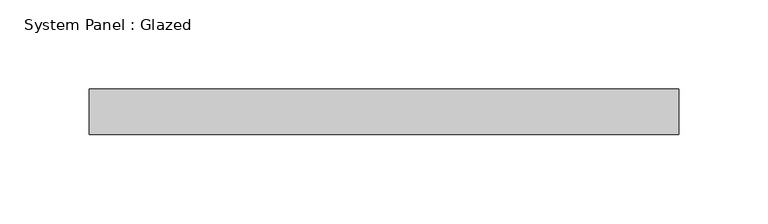
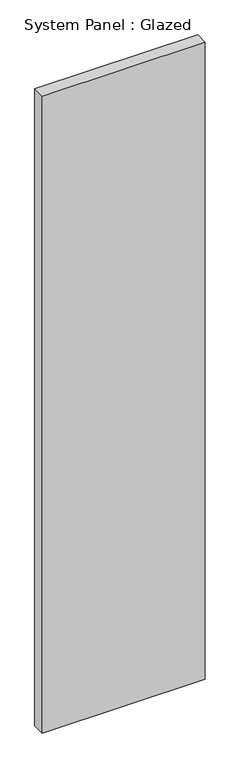
"""IFC4 building model written with IfcOpenShell, lengths in millimetres: plate geometry, System Panel : Glazed."""

from ifc_helpers import new_model, si_unit, origin, origin_with_axes, place, context, project, spatial, polyline, outline, extrude, source, transform, mapped, element, save


def system_panel_glazed_df80ca6a(model_context):
    return source(origin(), model_context, "Body", "SweptSolid", [
        extrude(outline(polyline([(165.1, 19.05), (-165.1, 19.05), (-165.1, 44.45), (165.1, 44.45), (165.1, 19.05)])), origin_with_axes(), (0.0, 0.0, 1.0), 1363.0142793),
    ])


if __name__ == "__main__":
    model = new_model("IFC4")
    model_context = context("Model", 3, world=origin())
    ifc_project = project(units=[si_unit("LENGTHUNIT", "METRE", prefix="MILLI")], contexts=[model_context])
    site = spatial("IfcSite", under=ifc_project)
    building = spatial("IfcBuilding", under=site)
    placement = place(None, origin())
    system_panel_glazed_shape = system_panel_glazed_df80ca6a(model_context)
    element("IfcPlate", 1, ObjectType="System Panel : Glazed", at=placement, inside=building, context=model_context, shape_type="MappedRepresentation", body=[
        mapped(system_panel_glazed_shape, transform((0.0, 0.0, 0.0), x_axis=(1.0, 0.0, 0.0), y_axis=(0.0, 1.0, 0.0), z_axis=(0.0, 0.0, 1.0))),
    ])
    save(model, "model.ifc")

# Revit data of these elements
# Type "System Panel : Glazed"
#   Construction Type Id = "GSP4R"
#   Analytic Construction = "1/8 in Pilkington single glazing"
#   Visual Light Transmittance = 0.9
#   Solar Heat Gain Coefficient = 0.86
#   Heat Transfer Coefficient (U) = 1.18115 BTU/(h·ft²·°F)
#   Define Thermal Properties by = 1
# Element 1 (IfcPlate, "System Panel : Glazed")
#   Materials on its faces: "Glass"
# Materials
#   "Glass": class "Glass", colour RGB 0 128 192, transparency 0.75, Description = "Soda Lime Glass", Cost = 0
